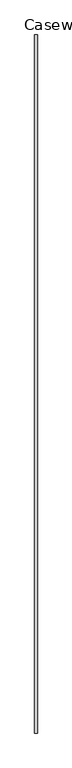
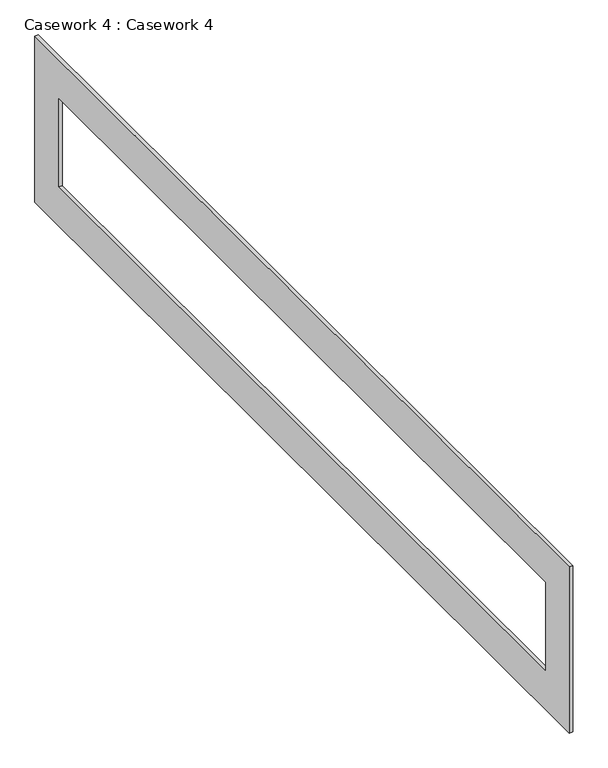
"""IFC4 building model written with IfcOpenShell, lengths in millimetres: furniture geometry, Casework 4 : Casework 4."""

from ifc_helpers import new_model, si_unit, frame, origin, place, context, project, spatial, polyline, outline, extrude, source, transform, mapped, element, save


def casework_4_casework_4_12d1038f(model_context):
    return source(origin(), model_context, "Body", "SweptSolid", [
        extrude(outline(polyline([(-1112.3742075, 7213.6), (-1112.3742075, 9809.0764163), (12552.8257925, 9809.0764163), (12552.8257925, 7213.6), (-1112.3742075, 7213.6)]), holes=[polyline([(-502.7742075, 7823.2), (11943.2257925, 7823.2), (11943.2257925, 9199.4764163), (-502.7742075, 9199.4764163), (-502.7742075, 7823.2)])]), frame((2710.0501403, 0.0, 0.0), z_axis=(1.0, 0.0, 0.0), x_axis=(0.0, 1.0, 0.0)), (0.0, 0.0, 1.0), 50.8),
    ])


if __name__ == "__main__":
    model = new_model("IFC4")
    model_context = context("Model", 3, world=origin())
    ifc_project = project(units=[si_unit("LENGTHUNIT", "METRE", prefix="MILLI")], contexts=[model_context])
    site = spatial("IfcSite", under=ifc_project)
    building = spatial("IfcBuilding", under=site)
    placement = place(None, origin())
    casework_4_casework_4_shape = casework_4_casework_4_12d1038f(model_context)
    element("IfcFurniture", 1, ObjectType="Casework 4 : Casework 4", at=placement, inside=building, context=model_context, shape_type="MappedRepresentation", body=[
        mapped(casework_4_casework_4_shape, transform((0.0, 0.0, 0.0), x_axis=(1.0, 0.0, 0.0), y_axis=(0.0, 1.0, 0.0), z_axis=(0.0, 0.0, 1.0))),
    ])
    save(model, "model.ifc")

# Revit data of these elements
# Element 1 (IfcFurniture, "Casework 4 : Casework 4")
#   Materials on its faces: "Linen, White"
# Materials
#   "Linen, White": class "Textile", colour RGB 247 247 239, transparency 0, Description = "Linen, white", Cost = 0
